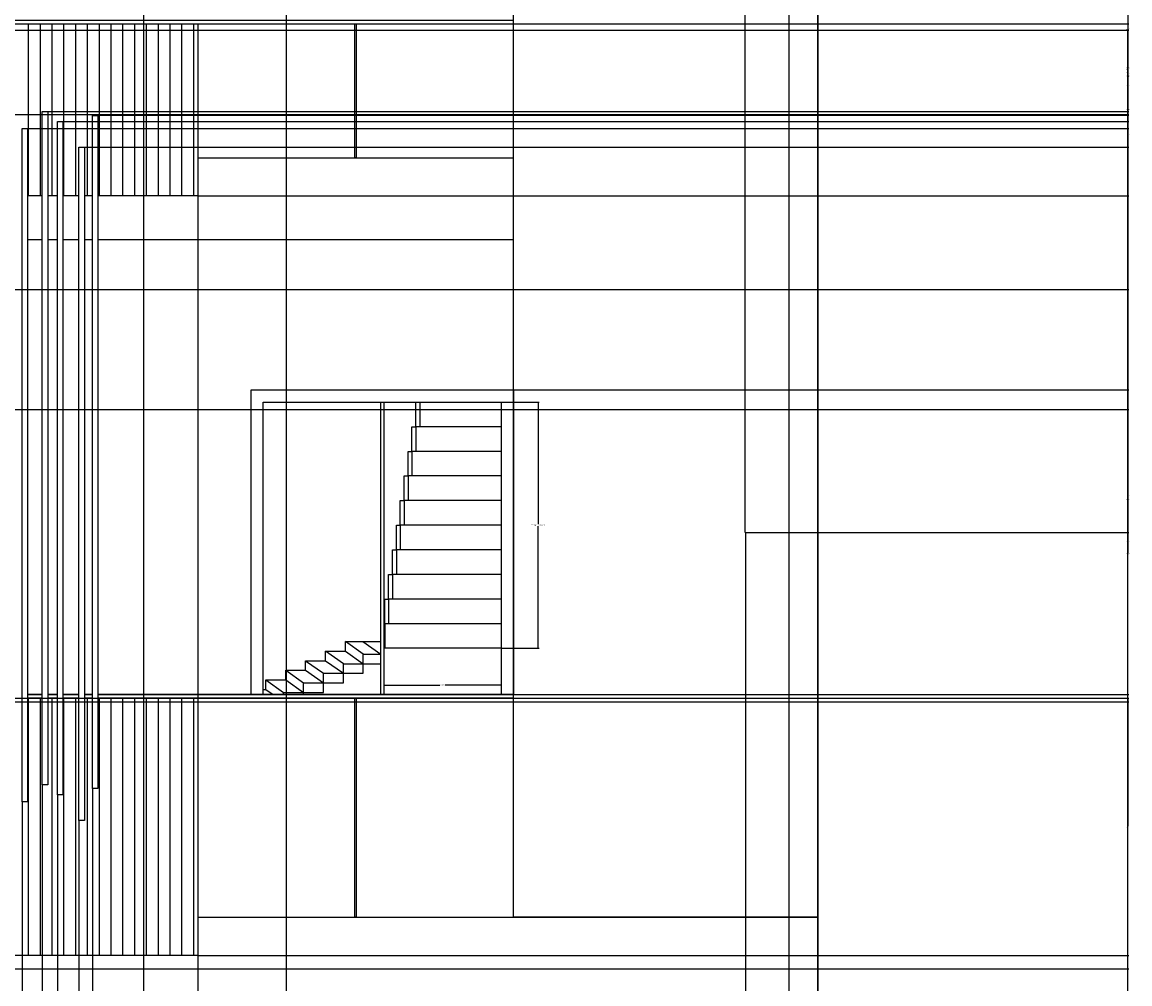
# Model space of a CAD drawing. Units: feet. Extents: x 2193 to 3502, y 890 to 1601.
# Tile 14 of 17: x 3281 to 3502, y 1076 to 1268. Entities that reach past the tile are written whole.
import ezdxf

# ---------------------------------------------------------------- set-up
doc = ezdxf.new("R2010")
doc.units = ezdxf.units.FT
doc.layers.add('A-ANNO-DIMS', color=2, linetype='Continuous', lineweight=18)
doc.layers.add('A-ELEV', color=7, linetype='Continuous', lineweight=25)
doc.styles.get("Standard").update_dxf_attribs({"font": 'arial.ttf'})
doc.dimstyles.get("Standard").update_dxf_attribs({"dimtxt": 0.18, "dimasz": 0.18, "dimexe": 0.18, "dimexo": 0.0625, "dimgap": 0.09, "dimtad": 0, "dimtih": 1, "dimtoh": 1, "dimdec": 0, "dimzin": 0, "dimdsep": 46, "dimlunit": 3, "dimtxsty": 'Standard', "dimcen": 0.09, "dimadec": 0, "dimazin": 0, "dimtfac": 1, "dimtdec": 0, "dimtofl": 0, "dimtmove": 0, "dimatfit": 3, "dimfxl": 1, "dimtolj": 1, "dimtzin": 0, "dimarcsym": 0})

# ---------------------------------------------------------------- blocks, each defined once
blk = doc.blocks.new('STAIR-RAIL-B')
for p, q in [((6.38, 44.29), (6.38, 49.22)), ((5.61, 39.37), (5.61, 44.29)), ((5.61, 44.29), (6.38, 44.29)), ((23.45, 44.29), (6.38, 44.29)), ((6.38, 44.29), (6.38, 39.37)), ((4.83, 34.45), (4.83, 39.37)), ((4.83, 39.37), (5.61, 39.37)), ((23.45, 39.37), (5.61, 39.37)), ((5.61, 39.37), (5.61, 34.45)), ((4.05, 29.53), (4.05, 34.45)), ((4.05, 34.45), (4.83, 34.45)), ((23.45, 34.45), (4.83, 34.45)), ((4.83, 34.45), (4.83, 29.53)), ((3.27, 24.61), (3.27, 29.53)), ((3.27, 29.53), (4.05, 29.53)), ((23.45, 29.53), (4.05, 29.53)), ((4.05, 29.53), (4.05, 24.61)), ((2.49, 19.69), (2.49, 24.61)), ((2.49, 24.61), (3.27, 24.61)), ((23.45, 24.61), (3.27, 24.61)), ((3.27, 24.61), (3.27, 19.69)), ((1.71, 14.77), (1.71, 19.69)), ((1.71, 19.69), (2.49, 19.69)), ((23.45, 19.69), (2.49, 19.69)), ((2.49, 19.69), (2.49, 14.77)), ((0.93, 9.84), (0.93, 14.77)), ((0.93, 14.77), (1.71, 14.77)), ((23.45, 14.77), (1.71, 14.77)), ((1.71, 14.77), (1.71, 9.84)), ((0.15, 4.92), (0.15, 9.84)), ((0.15, 9.84), (0.93, 9.84)), ((23.45, 9.84), (0.93, 9.84)), ((0.93, 9.84), (0.93, 4.92)), ((23.45, 4.92), (0, 4.92)), ((0.15, 4.92), (0.15, 0)), ((23.45, 0), (0, 0))]:
    blk.add_line(p, q)
blk = doc.blocks.new('*D9')
at = {"layer": 'A-ANNO-DIMS', "color": 0, "lineweight": -2, "transparency": 16777216}
for p, q in [((3376.47, 1192.33), (3383.97, 1192.33)), ((3383.79, 1192.15), (3383.79, 1167.9)), ((3383.79, 1143.29), (3383.79, 1167.54)), ((3376.47, 1143.11), (3383.97, 1143.11))]:
    blk.add_line(p, q, dxfattribs=at)
at = {"layer": 'A-ANNO-DIMS', "color": 0, "transparency": 16777216}
for points in [[(3383.76, 1192.15), (3383.82, 1192.15), (3383.79, 1192.33)], [(3383.76, 1143.29), (3383.82, 1143.29), (3383.79, 1143.11)]]:
    blk.add_solid(points, dxfattribs=at)
at = {"layer": 'Defpoints', "color": 0, "transparency": 16777216}
for p in [(3376.4, 1192.33), (3383.79, 1192.33), (3376.4, 1143.11)]:
    blk.add_point(p, dxfattribs=at)
at = {"layer": 'A-ANNO-DIMS', "color": 0, "transparency": 16777216, "insert": (3383.79, 1167.72), "char_height": 0.18, "attachment_point": 5}
blk.add_mtext('\\A1;STAIR RAILING B 49 TYP.', dxfattribs=at)
blk = doc.blocks.new('*D10')
at = {"layer": 'A-ANNO-DIMS', "color": 0, "lineweight": -2, "transparency": 16777216}
for p, q in [((3352.95, 1143.05), (3352.95, 1135.55)), ((3376.4, 1143.05), (3376.4, 1135.55)), ((3353.13, 1135.73), (3364.15, 1135.73)), ((3376.22, 1135.73), (3365.21, 1135.73))]:
    blk.add_line(p, q, dxfattribs=at)
at = {"layer": 'A-ANNO-DIMS', "color": 0, "transparency": 16777216}
for points in [[(3353.13, 1135.76), (3353.13, 1135.7), (3352.95, 1135.73)], [(3376.22, 1135.76), (3376.22, 1135.7), (3376.4, 1135.73)]]:
    blk.add_solid(points, dxfattribs=at)
at = {"layer": 'Defpoints', "color": 0, "transparency": 16777216}
for p in [(3352.95, 1143.11), (3376.4, 1143.11), (3376.4, 1135.73)]:
    blk.add_point(p, dxfattribs=at)
at = {"layer": 'A-ANNO-DIMS', "color": 0, "transparency": 16777216, "insert": (3364.68, 1135.73), "char_height": 0.18, "attachment_point": 5}
blk.add_mtext('\\A1;23 TYP.', dxfattribs=at)
blk = doc.blocks.new('*D13')
at = {"layer": 'A-ANNO-DIMS', "color": 0, "lineweight": -2, "transparency": 16777216}
for p, q in [((2934.37, 950.89), (2934.37, 1601.47)), ((2934.55, 1601.29), (3186.64, 1601.29)), ((3439.51, 1601.29), (3187.43, 1601.29)), ((3439.69, 1541.11), (3439.69, 1601.47))]:
    blk.add_line(p, q, dxfattribs=at)
at = {"layer": 'A-ANNO-DIMS', "color": 0, "transparency": 16777216}
for points in [[(2934.55, 1601.32), (2934.55, 1601.26), (2934.37, 1601.29)], [(3439.51, 1601.32), (3439.51, 1601.26), (3439.69, 1601.29)]]:
    blk.add_solid(points, dxfattribs=at)
at = {"layer": 'Defpoints', "color": 0, "transparency": 16777216}
for p in [(3439.69, 1601.29), (3439.69, 1541.04), (2934.37, 950.82)]:
    blk.add_point(p, dxfattribs=at)
at = {"layer": 'A-ANNO-DIMS', "color": 0, "transparency": 16777216, "insert": (3187.03, 1601.29), "char_height": 0.18, "attachment_point": 5}
blk.add_mtext('\\A1;505.3', dxfattribs=at)
blk = doc.blocks.new('*D18')
at = {"layer": 'A-ANNO-DIMS', "color": 0, "lineweight": -2, "transparency": 16777216}
for p, q in [((3439.75, 1541.04), (3501.85, 1541.04)), ((3501.67, 1540.86), (3501.67, 1246.12)), ((3501.67, 951), (3501.67, 1245.75)), ((3441.48, 950.82), (3501.85, 950.82))]:
    blk.add_line(p, q, dxfattribs=at)
at = {"layer": 'A-ANNO-DIMS', "color": 0, "transparency": 16777216}
for points in [[(3501.64, 1540.86), (3501.7, 1540.86), (3501.67, 1541.04)], [(3501.64, 951), (3501.7, 951), (3501.67, 950.82)]]:
    blk.add_solid(points, dxfattribs=at)
at = {"layer": 'Defpoints', "color": 0, "transparency": 16777216}
for p in [(3439.69, 1541.04), (3501.67, 1541.04), (3441.42, 950.82)]:
    blk.add_point(p, dxfattribs=at)
at = {"layer": 'A-ANNO-DIMS', "color": 0, "transparency": 16777216, "insert": (3501.67, 1245.93), "char_height": 0.18, "attachment_point": 5}
blk.add_mtext('\\A1;590.2', dxfattribs=at)
blk = doc.blocks.new('*D31')
at = {"layer": 'A-ANNO-DIMS', "color": 0, "lineweight": -2, "transparency": 16777216}
for p, q in [((2760.54, 1541.04), (3501.85, 1541.04)), ((3501.67, 1540.86), (3501.67, 1246.12)), ((3501.67, 951), (3501.67, 1245.75)), ((2762.27, 950.82), (3501.85, 950.82))]:
    blk.add_line(p, q, dxfattribs=at)
at = {"layer": 'A-ANNO-DIMS', "color": 0, "transparency": 16777216}
for points in [[(3501.64, 1540.86), (3501.7, 1540.86), (3501.67, 1541.04)], [(3501.64, 951), (3501.7, 951), (3501.67, 950.82)]]:
    blk.add_solid(points, dxfattribs=at)
at = {"layer": 'Defpoints', "color": 0, "transparency": 16777216}
for p in [(2760.47, 1541.04), (3501.67, 1541.04), (2762.2, 950.82)]:
    blk.add_point(p, dxfattribs=at)
at = {"layer": 'A-ANNO-DIMS', "color": 0, "transparency": 16777216, "insert": (3501.67, 1245.93), "char_height": 0.18, "attachment_point": 5}
blk.add_mtext('\\A1;590.2', dxfattribs=at)
blk = doc.blocks.new('*D62')
at = {"layer": 'A-ANNO-DIMS', "color": 0, "lineweight": -2, "transparency": 16777216}
for p, q in [((2974.18, 1266.71), (3501.85, 1266.71)), ((3501.67, 1266.53), (3501.67, 1173.05)), ((3501.67, 1079.21), (3501.67, 1172.69)), ((2974.18, 1079.03), (3501.85, 1079.03))]:
    blk.add_line(p, q, dxfattribs=at)
at = {"layer": 'A-ANNO-DIMS', "color": 0, "transparency": 16777216}
for points in [[(3501.64, 1266.53), (3501.7, 1266.53), (3501.67, 1266.71)], [(3501.64, 1079.21), (3501.7, 1079.21), (3501.67, 1079.03)]]:
    blk.add_solid(points, dxfattribs=at)
at = {"layer": 'Defpoints', "color": 0, "transparency": 16777216}
for p in [(2974.12, 1266.71), (3501.67, 1266.71), (2974.12, 1079.03)]:
    blk.add_point(p, dxfattribs=at)
at = {"layer": 'A-ANNO-DIMS', "color": 0, "transparency": 16777216, "insert": (3501.67, 1172.87), "char_height": 0.18, "attachment_point": 5}
blk.add_mtext('\\A1;187.68', dxfattribs=at)
blk = doc.blocks.new('*D67')
at = {"layer": 'A-ANNO-DIMS', "color": 0, "lineweight": -2, "transparency": 16777216}
for p, q in [((2980.78, 1214.84), (3501.85, 1214.84)), ((3501.67, 1214.66), (3501.67, 1173.8)), ((3501.67, 1132.57), (3501.67, 1173.43)), ((2980.78, 1132.39), (3501.85, 1132.39))]:
    blk.add_line(p, q, dxfattribs=at)
at = {"layer": 'A-ANNO-DIMS', "color": 0, "transparency": 16777216}
for points in [[(3501.64, 1214.66), (3501.7, 1214.66), (3501.67, 1214.84)], [(3501.64, 1132.57), (3501.7, 1132.57), (3501.67, 1132.39)]]:
    blk.add_solid(points, dxfattribs=at)
at = {"layer": 'Defpoints', "color": 0, "transparency": 16777216}
for p in [(2980.72, 1214.84), (3501.67, 1214.84), (2980.72, 1132.39)]:
    blk.add_point(p, dxfattribs=at)
at = {"layer": 'A-ANNO-DIMS', "color": 0, "transparency": 16777216, "insert": (3501.67, 1173.62), "char_height": 0.18, "attachment_point": 5}
blk.add_mtext('\\A1;82.44', dxfattribs=at)
blk = doc.blocks.new('*D69')
at = {"layer": 'A-ANNO-DIMS', "color": 0, "lineweight": -2, "transparency": 16777216}
for p, q in [((3425.25, 1367.57), (3501.85, 1367.57)), ((3501.67, 1367.39), (3501.67, 1267.09)), ((3501.67, 1166.41), (3501.67, 1266.72)), ((3425.25, 1166.23), (3501.85, 1166.23))]:
    blk.add_line(p, q, dxfattribs=at)
at = {"layer": 'A-ANNO-DIMS', "color": 0, "transparency": 16777216}
for points in [[(3501.64, 1367.39), (3501.7, 1367.39), (3501.67, 1367.57)], [(3501.64, 1166.41), (3501.7, 1166.41), (3501.67, 1166.23)]]:
    blk.add_solid(points, dxfattribs=at)
at = {"layer": 'Defpoints', "color": 0, "transparency": 16777216}
for p in [(3425.19, 1367.57), (3501.67, 1367.57), (3425.19, 1166.23)]:
    blk.add_point(p, dxfattribs=at)
at = {"layer": 'A-ANNO-DIMS', "color": 0, "transparency": 16777216, "insert": (3501.67, 1266.9), "char_height": 0.18, "attachment_point": 5}
blk.add_mtext('\\A1;201.34', dxfattribs=at)
blk = doc.blocks.new('*D70')
at = {"layer": 'A-ANNO-DIMS', "color": 0, "lineweight": -2, "transparency": 16777216}
for p, q in [((3425.19, 1166.17), (3425.19, 890.39)), ((3439.69, 1166.17), (3439.69, 890.39)), ((3425.37, 890.57), (3431.98, 890.57)), ((3439.51, 890.57), (3432.89, 890.57))]:
    blk.add_line(p, q, dxfattribs=at)
at = {"layer": 'A-ANNO-DIMS', "color": 0, "transparency": 16777216}
for points in [[(3425.37, 890.6), (3425.37, 890.54), (3425.19, 890.57)], [(3439.51, 890.6), (3439.51, 890.54), (3439.69, 890.57)]]:
    blk.add_solid(points, dxfattribs=at)
at = {"layer": 'Defpoints', "color": 0, "transparency": 16777216}
for p in [(3425.19, 1166.23), (3439.69, 1166.23), (3439.69, 890.57)]:
    blk.add_point(p, dxfattribs=at)
at = {"layer": 'A-ANNO-DIMS', "color": 0, "transparency": 16777216, "insert": (3432.44, 890.57), "char_height": 0.18, "attachment_point": 5}
blk.add_mtext('\\A1;14.502', dxfattribs=at)
blk = doc.blocks.new('*D76')
at = {"layer": 'A-ANNO-DIMS', "color": 0, "lineweight": -2, "transparency": 16777216}
for p, q in [((3259.05, 1190.87), (3501.85, 1190.87)), ((3501.67, 1190.69), (3501.67, 1162.17)), ((3501.67, 1133.29), (3501.67, 1161.81)), ((3259.52, 1133.11), (3501.85, 1133.11))]:
    blk.add_line(p, q, dxfattribs=at)
at = {"layer": 'A-ANNO-DIMS', "color": 0, "transparency": 16777216}
for points in [[(3501.64, 1190.69), (3501.7, 1190.69), (3501.67, 1190.87)], [(3501.64, 1133.29), (3501.7, 1133.29), (3501.67, 1133.11)]]:
    blk.add_solid(points, dxfattribs=at)
at = {"layer": 'Defpoints', "color": 0, "transparency": 16777216}
for p in [(3258.98, 1190.87), (3501.67, 1190.87), (3259.46, 1133.11)]:
    blk.add_point(p, dxfattribs=at)
at = {"layer": 'A-ANNO-DIMS', "color": 0, "transparency": 16777216, "insert": (3501.67, 1161.99), "char_height": 0.18, "attachment_point": 5}
blk.add_mtext('\\A1;57.75', dxfattribs=at)
blk = doc.blocks.new('*D79')
at = {"layer": 'A-ANNO-DIMS', "color": 0, "lineweight": -2, "transparency": 16777216}
for p, q in [((3326.46, 1194.77), (3501.85, 1194.77)), ((3501.67, 1194.59), (3501.67, 1164.5)), ((3501.67, 1134.04), (3501.67, 1164.13)), ((3326.46, 1133.86), (3501.85, 1133.86))]:
    blk.add_line(p, q, dxfattribs=at)
at = {"layer": 'A-ANNO-DIMS', "color": 0, "transparency": 16777216}
for points in [[(3501.64, 1194.59), (3501.7, 1194.59), (3501.67, 1194.77)], [(3501.64, 1134.04), (3501.7, 1134.04), (3501.67, 1133.86)]]:
    blk.add_solid(points, dxfattribs=at)
at = {"layer": 'Defpoints', "color": 0, "transparency": 16777216}
for p in [(3326.4, 1194.77), (3501.67, 1194.77), (3326.4, 1133.86)]:
    blk.add_point(p, dxfattribs=at)
at = {"layer": 'A-ANNO-DIMS', "color": 0, "transparency": 16777216, "insert": (3501.67, 1164.31), "char_height": 0.18, "attachment_point": 5}
blk.add_mtext('\\A1;60.92', dxfattribs=at)
blk = doc.blocks.new('*D80')
at = {"layer": 'A-ANNO-DIMS', "color": 0, "lineweight": -2, "transparency": 16777216}
for p, q in [((3198.15, 1233.5), (3198.15, 890.39)), ((3315.74, 1233.5), (3315.74, 890.39)), ((3198.33, 890.57), (3256.49, 890.57)), ((3315.56, 890.57), (3257.4, 890.57))]:
    blk.add_line(p, q, dxfattribs=at)
at = {"layer": 'A-ANNO-DIMS', "color": 0, "transparency": 16777216}
for points in [[(3198.33, 890.6), (3198.33, 890.54), (3198.15, 890.57)], [(3315.56, 890.6), (3315.56, 890.54), (3315.74, 890.57)]]:
    blk.add_solid(points, dxfattribs=at)
at = {"layer": 'Defpoints', "color": 0, "transparency": 16777216}
for p in [(3198.15, 1233.56), (3315.74, 1233.56), (3315.74, 890.57)]:
    blk.add_point(p, dxfattribs=at)
at = {"layer": 'A-ANNO-DIMS', "color": 0, "transparency": 16777216, "insert": (3256.94, 890.57), "char_height": 0.18, "attachment_point": 5}
blk.add_mtext('\\A1;117.58', dxfattribs=at)
blk = doc.blocks.new('*D81')
at = {"layer": 'A-ANNO-DIMS', "color": 0, "lineweight": -2, "transparency": 16777216}
for p, q in [((3315.8, 1267.92), (3501.85, 1267.92)), ((3501.67, 1267.74), (3501.67, 1250.92)), ((3501.67, 1233.74), (3501.67, 1250.56)), ((3315.8, 1233.56), (3501.85, 1233.56))]:
    blk.add_line(p, q, dxfattribs=at)
at = {"layer": 'A-ANNO-DIMS', "color": 0, "transparency": 16777216}
for points in [[(3501.64, 1267.74), (3501.7, 1267.74), (3501.67, 1267.92)], [(3501.64, 1233.74), (3501.7, 1233.74), (3501.67, 1233.56)]]:
    blk.add_solid(points, dxfattribs=at)
at = {"layer": 'Defpoints', "color": 0, "transparency": 16777216}
for p in [(3315.74, 1267.92), (3501.67, 1267.92), (3315.74, 1233.56)]:
    blk.add_point(p, dxfattribs=at)
at = {"layer": 'A-ANNO-DIMS', "color": 0, "transparency": 16777216, "insert": (3501.67, 1250.74), "char_height": 0.18, "attachment_point": 5}
blk.add_mtext('\\A1;34.356', dxfattribs=at)
blk = doc.blocks.new('*D82')
at = {"layer": 'A-ANNO-DIMS', "color": 0, "lineweight": -2, "transparency": 16777216}
for p, q in [((3315.8, 1133.11), (3501.85, 1133.11)), ((3501.67, 1132.93), (3501.67, 1107.6)), ((3501.67, 1081.91), (3501.67, 1107.24)), ((3315.8, 1081.73), (3501.85, 1081.73))]:
    blk.add_line(p, q, dxfattribs=at)
at = {"layer": 'A-ANNO-DIMS', "color": 0, "transparency": 16777216}
for points in [[(3501.64, 1132.93), (3501.7, 1132.93), (3501.67, 1133.11)], [(3501.64, 1081.91), (3501.7, 1081.91), (3501.67, 1081.73)]]:
    blk.add_solid(points, dxfattribs=at)
at = {"layer": 'Defpoints', "color": 0, "transparency": 16777216}
for p in [(3315.74, 1133.11), (3501.67, 1133.11), (3315.74, 1081.73)]:
    blk.add_point(p, dxfattribs=at)
at = {"layer": 'A-ANNO-DIMS', "color": 0, "transparency": 16777216, "insert": (3501.67, 1107.42), "char_height": 0.18, "attachment_point": 5}
blk.add_mtext('\\A1;51.39', dxfattribs=at)
blk = doc.blocks.new('*D86')
at = {"layer": 'A-ANNO-DIMS', "color": 0, "lineweight": -2, "transparency": 16777216}
for p, q in [((3277.81, 1115.17), (3277.81, 890.39)), ((3280.64, 1112.39), (3280.64, 890.39)), ((3277.99, 890.57), (3278.83, 890.57)), ((3280.46, 890.57), (3279.62, 890.57))]:
    blk.add_line(p, q, dxfattribs=at)
at = {"layer": 'A-ANNO-DIMS', "color": 0, "transparency": 16777216}
for points in [[(3277.99, 890.6), (3277.99, 890.54), (3277.81, 890.57)], [(3280.46, 890.6), (3280.46, 890.54), (3280.64, 890.57)]]:
    blk.add_solid(points, dxfattribs=at)
at = {"layer": 'Defpoints', "color": 0, "transparency": 16777216}
for p in [(3277.81, 1115.23), (3280.64, 1112.45), (3280.64, 890.57)]:
    blk.add_point(p, dxfattribs=at)
at = {"layer": 'A-ANNO-DIMS', "color": 0, "transparency": 16777216, "insert": (3279.22, 890.57), "char_height": 0.18, "attachment_point": 5}
blk.add_mtext('\\A1;2.832', dxfattribs=at)
blk = doc.blocks.new('*D87')
at = {"layer": 'A-ANNO-DIMS', "color": 0, "lineweight": -2, "transparency": 16777216}
for p, q in [((3284.65, 1115.79), (3284.65, 890.39)), ((3280.64, 1112.39), (3280.64, 890.39)), ((3280.82, 890.57), (3282.27, 890.57)), ((3284.47, 890.57), (3283.03, 890.57))]:
    blk.add_line(p, q, dxfattribs=at)
at = {"layer": 'A-ANNO-DIMS', "color": 0, "transparency": 16777216}
for points in [[(3280.82, 890.6), (3280.82, 890.54), (3280.64, 890.57)], [(3284.47, 890.6), (3284.47, 890.54), (3284.65, 890.57)]]:
    blk.add_solid(points, dxfattribs=at)
at = {"layer": 'Defpoints', "color": 0, "transparency": 16777216}
for p in [(3284.65, 1115.85), (3280.64, 1112.45), (3284.65, 890.57)]:
    blk.add_point(p, dxfattribs=at)
at = {"layer": 'A-ANNO-DIMS', "color": 0, "transparency": 16777216, "insert": (3282.65, 890.57), "char_height": 0.18, "attachment_point": 5}
blk.add_mtext('\\A1;4.011', dxfattribs=at)
blk = doc.blocks.new('*D88')
at = {"layer": 'A-ANNO-DIMS', "color": 0, "lineweight": -2, "transparency": 16777216}
for p, q in [((3284.65, 1115.79), (3284.65, 890.39)), ((3287.7, 1113.78), (3287.7, 890.39)), ((3284.83, 890.57), (3285.78, 890.57)), ((3287.52, 890.57), (3286.57, 890.57))]:
    blk.add_line(p, q, dxfattribs=at)
at = {"layer": 'A-ANNO-DIMS', "color": 0, "transparency": 16777216}
for points in [[(3284.83, 890.6), (3284.83, 890.54), (3284.65, 890.57)], [(3287.52, 890.6), (3287.52, 890.54), (3287.7, 890.57)]]:
    blk.add_solid(points, dxfattribs=at)
at = {"layer": 'Defpoints', "color": 0, "transparency": 16777216}
for p in [(3284.65, 1115.85), (3287.7, 1113.84), (3287.7, 890.57)]:
    blk.add_point(p, dxfattribs=at)
at = {"layer": 'A-ANNO-DIMS', "color": 0, "transparency": 16777216, "insert": (3286.18, 890.57), "char_height": 0.18, "attachment_point": 5}
blk.add_mtext('\\A1;3.052', dxfattribs=at)
blk = doc.blocks.new('*D89')
at = {"layer": 'A-ANNO-DIMS', "color": 0, "lineweight": -2, "transparency": 16777216}
for p, q in [((3287.7, 1113.78), (3287.7, 890.39)), ((3291.98, 1108.64), (3291.98, 890.39)), ((3287.88, 890.57), (3289.44, 890.57)), ((3291.8, 890.57), (3290.24, 890.57))]:
    blk.add_line(p, q, dxfattribs=at)
at = {"layer": 'A-ANNO-DIMS', "color": 0, "transparency": 16777216}
for points in [[(3287.88, 890.6), (3287.88, 890.54), (3287.7, 890.57)], [(3291.8, 890.6), (3291.8, 890.54), (3291.98, 890.57)]]:
    blk.add_solid(points, dxfattribs=at)
at = {"layer": 'Defpoints', "color": 0, "transparency": 16777216}
for p in [(3287.7, 1113.84), (3291.98, 1108.7), (3291.98, 890.57)]:
    blk.add_point(p, dxfattribs=at)
at = {"layer": 'A-ANNO-DIMS', "color": 0, "transparency": 16777216, "insert": (3289.84, 890.57), "char_height": 0.18, "attachment_point": 5}
blk.add_mtext('\\A1;4.273', dxfattribs=at)
blk = doc.blocks.new('*D90')
at = {"layer": 'A-ANNO-DIMS', "color": 0, "lineweight": -2, "transparency": 16777216}
for p, q in [((3294.68, 1115), (3294.68, 890.39)), ((3291.98, 1108.64), (3291.98, 890.39)), ((3292.16, 890.57), (3292.93, 890.57)), ((3294.5, 890.57), (3293.72, 890.57))]:
    blk.add_line(p, q, dxfattribs=at)
at = {"layer": 'A-ANNO-DIMS', "color": 0, "transparency": 16777216}
for points in [[(3292.16, 890.6), (3292.16, 890.54), (3291.98, 890.57)], [(3294.5, 890.6), (3294.5, 890.54), (3294.68, 890.57)]]:
    blk.add_solid(points, dxfattribs=at)
at = {"layer": 'Defpoints', "color": 0, "transparency": 16777216}
for p in [(3294.68, 1115.06), (3291.98, 1108.7), (3294.68, 890.57)]:
    blk.add_point(p, dxfattribs=at)
at = {"layer": 'A-ANNO-DIMS', "color": 0, "transparency": 16777216, "insert": (3293.33, 890.57), "char_height": 0.18, "attachment_point": 5}
blk.add_mtext('\\A1;2.703', dxfattribs=at)
blk = doc.blocks.new('*D91')
at = {"layer": 'A-ANNO-DIMS', "color": 0, "lineweight": -2, "transparency": 16777216}
for p, q in [((3277.2, 1267.92), (3501.85, 1267.92)), ((3501.67, 1267.74), (3501.67, 1259.05)), ((3501.67, 1250.01), (3501.67, 1258.69)), ((3277.87, 1249.83), (3501.85, 1249.83))]:
    blk.add_line(p, q, dxfattribs=at)
at = {"layer": 'A-ANNO-DIMS', "color": 0, "transparency": 16777216}
for points in [[(3501.64, 1267.74), (3501.7, 1267.74), (3501.67, 1267.92)], [(3501.64, 1250.01), (3501.7, 1250.01), (3501.67, 1249.83)]]:
    blk.add_solid(points, dxfattribs=at)
at = {"layer": 'Defpoints', "color": 0, "transparency": 16777216}
for p in [(3277.14, 1267.92), (3501.67, 1267.92), (3277.81, 1249.83)]:
    blk.add_point(p, dxfattribs=at)
at = {"layer": 'A-ANNO-DIMS', "color": 0, "transparency": 16777216, "insert": (3501.67, 1258.87), "char_height": 0.18, "attachment_point": 5}
blk.add_mtext('\\A1;18.09', dxfattribs=at)
blk = doc.blocks.new('*D92')
at = {"layer": 'A-ANNO-DIMS', "color": 0, "lineweight": -2, "transparency": 16777216}
for p, q in [((3281.92, 1267.92), (3501.85, 1267.92)), ((3501.67, 1267.74), (3501.67, 1257.66)), ((3501.67, 1247.22), (3501.67, 1257.3)), ((3280.7, 1247.04), (3501.85, 1247.04))]:
    blk.add_line(p, q, dxfattribs=at)
at = {"layer": 'A-ANNO-DIMS', "color": 0, "transparency": 16777216}
for points in [[(3501.64, 1267.74), (3501.7, 1267.74), (3501.67, 1267.92)], [(3501.64, 1247.22), (3501.7, 1247.22), (3501.67, 1247.04)]]:
    blk.add_solid(points, dxfattribs=at)
at = {"layer": 'Defpoints', "color": 0, "transparency": 16777216}
for p in [(3281.86, 1267.92), (3501.67, 1267.92), (3280.64, 1247.04)]:
    blk.add_point(p, dxfattribs=at)
at = {"layer": 'A-ANNO-DIMS', "color": 0, "transparency": 16777216, "insert": (3501.67, 1257.48), "char_height": 0.18, "attachment_point": 5}
blk.add_mtext('\\A1;20.875', dxfattribs=at)
blk = doc.blocks.new('*D93')
at = {"layer": 'A-ANNO-DIMS', "color": 0, "lineweight": -2, "transparency": 16777216}
for p, q in [((3284.28, 1267.92), (3501.85, 1267.92)), ((3501.67, 1267.74), (3501.67, 1259.36)), ((3501.67, 1250.62), (3501.67, 1259)), ((3284.71, 1250.44), (3501.85, 1250.44))]:
    blk.add_line(p, q, dxfattribs=at)
at = {"layer": 'A-ANNO-DIMS', "color": 0, "transparency": 16777216}
for points in [[(3501.64, 1267.74), (3501.7, 1267.74), (3501.67, 1267.92)], [(3501.64, 1250.62), (3501.7, 1250.62), (3501.67, 1250.44)]]:
    blk.add_solid(points, dxfattribs=at)
at = {"layer": 'Defpoints', "color": 0, "transparency": 16777216}
for p in [(3284.22, 1267.92), (3501.67, 1267.92), (3284.65, 1250.44)]:
    blk.add_point(p, dxfattribs=at)
at = {"layer": 'A-ANNO-DIMS', "color": 0, "transparency": 16777216, "insert": (3501.67, 1259.18), "char_height": 0.18, "attachment_point": 5}
blk.add_mtext('\\A1;17.477', dxfattribs=at)
blk = doc.blocks.new('*D94')
at = {"layer": 'A-ANNO-DIMS', "color": 0, "lineweight": -2, "transparency": 16777216}
for p, q in [((3288.99, 1267.92), (3501.85, 1267.92)), ((3501.67, 1267.74), (3501.67, 1258.36)), ((3501.67, 1248.62), (3501.67, 1257.99)), ((3287.77, 1248.44), (3501.85, 1248.44))]:
    blk.add_line(p, q, dxfattribs=at)
at = {"layer": 'A-ANNO-DIMS', "color": 0, "transparency": 16777216}
for points in [[(3501.64, 1267.74), (3501.7, 1267.74), (3501.67, 1267.92)], [(3501.64, 1248.62), (3501.7, 1248.62), (3501.67, 1248.44)]]:
    blk.add_solid(points, dxfattribs=at)
at = {"layer": 'Defpoints', "color": 0, "transparency": 16777216}
for p in [(3288.93, 1267.92), (3501.67, 1267.92), (3287.7, 1248.44)]:
    blk.add_point(p, dxfattribs=at)
at = {"layer": 'A-ANNO-DIMS', "color": 0, "transparency": 16777216, "insert": (3501.67, 1258.18), "char_height": 0.18, "attachment_point": 5}
blk.add_mtext('\\A1;19.48', dxfattribs=at)
blk = doc.blocks.new('*D95')
at = {"layer": 'A-ANNO-DIMS', "color": 0, "lineweight": -2, "transparency": 16777216}
for p, q in [((3291.35, 1267.92), (3501.85, 1267.92)), ((3501.67, 1267.74), (3501.67, 1255.79)), ((3501.67, 1243.48), (3501.67, 1255.42)), ((3292.04, 1243.3), (3501.85, 1243.3))]:
    blk.add_line(p, q, dxfattribs=at)
at = {"layer": 'A-ANNO-DIMS', "color": 0, "transparency": 16777216}
for points in [[(3501.64, 1267.74), (3501.7, 1267.74), (3501.67, 1267.92)], [(3501.64, 1243.48), (3501.7, 1243.48), (3501.67, 1243.3)]]:
    blk.add_solid(points, dxfattribs=at)
at = {"layer": 'Defpoints', "color": 0, "transparency": 16777216}
for p in [(3291.29, 1267.92), (3501.67, 1267.92), (3291.98, 1243.3)]:
    blk.add_point(p, dxfattribs=at)
at = {"layer": 'A-ANNO-DIMS', "color": 0, "transparency": 16777216, "insert": (3501.67, 1255.61), "char_height": 0.18, "attachment_point": 5}
blk.add_mtext('\\A1;24.62', dxfattribs=at)
blk = doc.blocks.new('*D96')
at = {"layer": 'A-ANNO-DIMS', "color": 0, "lineweight": -2, "transparency": 16777216}
for p, q in [((3296.07, 1267.92), (3501.85, 1267.92)), ((3501.67, 1267.74), (3501.67, 1258.97)), ((3501.67, 1249.84), (3501.67, 1258.6)), ((3294.74, 1249.66), (3501.85, 1249.66))]:
    blk.add_line(p, q, dxfattribs=at)
at = {"layer": 'A-ANNO-DIMS', "color": 0, "transparency": 16777216}
for points in [[(3501.64, 1267.74), (3501.7, 1267.74), (3501.67, 1267.92)], [(3501.64, 1249.84), (3501.7, 1249.84), (3501.67, 1249.66)]]:
    blk.add_solid(points, dxfattribs=at)
at = {"layer": 'Defpoints', "color": 0, "transparency": 16777216}
for p in [(3296, 1267.92), (3501.67, 1267.92), (3294.68, 1249.66)]:
    blk.add_point(p, dxfattribs=at)
at = {"layer": 'A-ANNO-DIMS', "color": 0, "transparency": 16777216, "insert": (3501.67, 1258.79), "char_height": 0.18, "attachment_point": 5}
blk.add_mtext('\\A1;18.26', dxfattribs=at)
blk = doc.blocks.new('*D97')
at = {"layer": 'A-ANNO-DIMS', "color": 0, "lineweight": -2, "transparency": 16777216}
for p, q in [((3111.13, 1032.26), (3111.13, 1601.47)), ((3111.31, 1601.29), (3207.6, 1601.29)), ((3304.79, 1601.29), (3208.51, 1601.29)), ((3304.97, 1032.26), (3304.97, 1601.47))]:
    blk.add_line(p, q, dxfattribs=at)
at = {"layer": 'A-ANNO-DIMS', "color": 0, "transparency": 16777216}
for points in [[(3111.31, 1601.32), (3111.31, 1601.26), (3111.13, 1601.29)], [(3304.79, 1601.32), (3304.79, 1601.26), (3304.97, 1601.29)]]:
    blk.add_solid(points, dxfattribs=at)
at = {"layer": 'Defpoints', "color": 0, "transparency": 16777216}
for p in [(3304.97, 1601.29), (3111.13, 1032.19), (3304.97, 1032.19)]:
    blk.add_point(p, dxfattribs=at)
at = {"layer": 'A-ANNO-DIMS', "color": 0, "transparency": 16777216, "insert": (3208.05, 1601.29), "char_height": 0.18, "attachment_point": 5}
blk.add_mtext('\\A1;193.84', dxfattribs=at)
blk = doc.blocks.new('*D123')
at = {"layer": 'A-ANNO-DIMS', "color": 0, "lineweight": -2, "transparency": 16777216}
for p, q in [((3433.98, 1073.09), (3433.98, 1601.47)), ((3434.16, 1601.29), (3436.44, 1601.29)), ((3439.51, 1601.29), (3437.23, 1601.29)), ((3439.69, 1073.09), (3439.69, 1601.47))]:
    blk.add_line(p, q, dxfattribs=at)
at = {"layer": 'A-ANNO-DIMS', "color": 0, "transparency": 16777216}
for points in [[(3434.16, 1601.32), (3434.16, 1601.26), (3433.98, 1601.29)], [(3439.51, 1601.32), (3439.51, 1601.26), (3439.69, 1601.29)]]:
    blk.add_solid(points, dxfattribs=at)
at = {"layer": 'Defpoints', "color": 0, "transparency": 16777216}
for p in [(3439.69, 1601.29), (3433.98, 1073.03), (3439.69, 1073.03)]:
    blk.add_point(p, dxfattribs=at)
at = {"layer": 'A-ANNO-DIMS', "color": 0, "transparency": 16777216, "insert": (3436.84, 1601.29), "char_height": 0.18, "attachment_point": 5}
blk.add_mtext('\\A1;5.707', dxfattribs=at)
blk = doc.blocks.new('*D125')
at = {"layer": 'A-ANNO-DIMS', "color": 0, "lineweight": -2, "transparency": 16777216}
for p, q in [((3304.97, 1073.09), (3304.97, 1601.47)), ((3305.15, 1601.29), (3318.84, 1601.29)), ((3333.32, 1601.29), (3319.63, 1601.29)), ((3333.5, 1073.09), (3333.5, 1601.47))]:
    blk.add_line(p, q, dxfattribs=at)
at = {"layer": 'A-ANNO-DIMS', "color": 0, "transparency": 16777216}
for points in [[(3305.15, 1601.32), (3305.15, 1601.26), (3304.97, 1601.29)], [(3333.32, 1601.32), (3333.32, 1601.26), (3333.5, 1601.29)]]:
    blk.add_solid(points, dxfattribs=at)
at = {"layer": 'Defpoints', "color": 0, "transparency": 16777216}
for p in [(3333.5, 1601.29), (3304.97, 1073.03), (3333.5, 1073.03)]:
    blk.add_point(p, dxfattribs=at)
at = {"layer": 'A-ANNO-DIMS', "color": 0, "transparency": 16777216, "insert": (3319.24, 1601.29), "char_height": 0.18, "attachment_point": 5}
blk.add_mtext('\\A1;28.53', dxfattribs=at)

msp = doc.modelspace()

# ---------------------------------------------------------------- linework, layer by layer
at = {"layer": 'A-ELEV'}
for p, q in [((3439.6901, 956.8829), (3439.6901, 1494.0584)), ((3315.7352, 1241.1967), (3378.849, 1241.1967)), ((3281.7371, 1224.865), (3284.651, 1224.865)), ((3285.7483, 1224.865), (3287.703, 1224.865)), ((3288.8003, 1224.865), (3291.9757, 1224.865)), ((3293.0731, 1224.865), (3294.679, 1224.865)), ((3295.7763, 1224.865), (3378.849, 1224.865)), ((3360.1133, 1192.3273), (3360.1133, 1187.4057)), ((3425.1877, 1166.2327), (3439.6901, 1166.2327)), ((3341.2875, 1140.6364), (3341.2875, 1142.554)), ((3341.2875, 1142.554), (3345.27, 1142.554)), ((3344.8379, 1140.0352), (3341.2875, 1142.554)), ((3348.8205, 1141.9528), (3345.27, 1144.4716)), ((3345.27, 1144.4716), (3348.7495, 1144.4716)), ((3345.27, 1142.554), (3345.27, 1144.4716)), ((3345.27, 1142.554), (3348.8205, 1140.0352)), ((3348.7495, 1144.4716), (3352.2999, 1141.9528)), ((3348.7495, 1144.4716), (3352.2999, 1144.4716)), ((3337.3049, 1138.7188), (3337.3049, 1140.6364)), ((3337.3049, 1140.6364), (3341.2875, 1140.6364)), ((3337.3049, 1140.6364), (3340.8553, 1138.1177)), ((3341.2875, 1140.6364), (3344.8379, 1138.1177)), ((3348.8205, 1140.0352), (3348.8205, 1141.9528)), ((3348.8205, 1141.9528), (3352.2999, 1141.9528)), ((3333.3223, 1136.8013), (3333.3223, 1138.7188)), ((3333.3223, 1138.7188), (3337.3049, 1138.7188)), ((3333.3223, 1138.7188), (3336.8727, 1136.2001)), ((3337.3049, 1138.7188), (3340.8553, 1136.2001)), ((3340.8553, 1136.2001), (3340.8553, 1138.1177)), ((3340.8553, 1138.1177), (3344.8379, 1138.1177)), ((3344.8379, 1138.1177), (3344.8379, 1140.0352)), ((3344.8379, 1140.0352), (3348.8205, 1140.0352)), ((3344.8379, 1136.2001), (3344.8379, 1138.1177)), ((3344.8379, 1138.1177), (3348.8205, 1138.1177)), ((3348.8205, 1140.0352), (3352.2999, 1140.0352)), ((3348.8205, 1138.1177), (3348.8205, 1140.0352)), ((3329.3397, 1134.8837), (3329.3397, 1136.8013)), ((3329.3397, 1136.8013), (3333.3223, 1136.8013)), ((3329.3397, 1136.8013), (3332.8902, 1134.2825)), ((3333.3223, 1136.8013), (3336.8727, 1134.2825)), ((3336.8727, 1134.2825), (3336.8727, 1136.2001)), ((3336.8727, 1136.2001), (3340.8553, 1136.2001)), ((3340.8553, 1134.2825), (3340.8553, 1136.2001)), ((3340.8553, 1136.2001), (3344.8379, 1136.2001)), ((3328.846, 1134.8837), (3329.3397, 1134.8837)), ((3329.3397, 1134.8837), (3330.7886, 1133.8558)), ((3332.8902, 1133.8558), (3332.8902, 1134.2825)), ((3332.8902, 1134.2825), (3336.8727, 1134.2825)), ((3332.8902, 1133.8558), (3332.8902, 1133.8558)), ((3336.8727, 1133.8558), (3336.8727, 1134.2825)), ((3336.8727, 1134.2825), (3340.8553, 1134.2825)), ((3315.7352, 1089.3627), (3439.6901, 1089.3627))]:
    msp.add_line(p, q, dxfattribs=at)
for points in [[(3439.6901, 1415.3157), (3439.6901, 1089.3627), (3378.849, 1089.3627), (3378.849, 1367.5739)], [(3425.1877, 1166.2327), (3425.1877, 1367.5739)], [(3378.849, 1267.9169), (3147.5022, 1267.9169), (3147.5022, 1268.6599), (3378.849, 1268.6599)], [(3281.8579, 1267.9169), (3281.8579, 1233.561), (3281.7371, 1233.561)], [(3284.2158, 1267.9169), (3284.2158, 1233.561), (3283.0369, 1233.561)], [(3286.5736, 1267.9169), (3286.5736, 1233.561), (3285.7483, 1233.561)], [(3288.9314, 1267.9169), (3288.9314, 1233.561), (3288.8003, 1233.561)], [(3291.2893, 1267.9169), (3291.2893, 1233.561), (3290.1104, 1233.561)], [(3293.6471, 1267.9169), (3293.6471, 1233.561), (3293.0731, 1233.561)], [(3315.7352, 1267.9169), (3315.7352, 1233.561), (3295.7763, 1233.561)], [(3296.005, 1267.9169), (3296.005, 1233.561), (3295.7763, 1233.561)], [(3298.3628, 1267.9169), (3298.3628, 1233.561), (3297.1839, 1233.561)], [(3300.7206, 1267.9169), (3300.7206, 1233.561), (3299.5417, 1233.561)], [(3303.0785, 1267.9169), (3303.0785, 1233.561), (3301.8996, 1233.561)], [(3305.4363, 1267.9169), (3305.4363, 1233.561), (3304.2574, 1233.561)], [(3307.7941, 1267.9169), (3307.7941, 1233.561), (3306.6152, 1233.561)], [(3310.152, 1267.9169), (3310.152, 1233.561), (3308.9731, 1233.561)], [(3312.5098, 1267.9169), (3312.5098, 1233.561), (3311.3309, 1233.561)], [(3314.8677, 1267.9169), (3314.8677, 1233.561), (3313.6887, 1233.561)], [(3347.39, 1267.9169), (3347.39, 1241.1967), (3347.1403, 1241.1967), (3347.1403, 1267.9169)], [(3284.651, 1233.561), (3281.7371, 1233.561)], [(3287.703, 1233.561), (3285.7483, 1233.561)], [(3291.9757, 1233.561), (3288.8003, 1233.561)], [(3294.679, 1233.561), (3293.0731, 1233.561)], [(3328.846, 1133.8558), (3328.846, 1192.3273), (3376.4039, 1192.3273), (3376.4039, 1133.8558)], [(3281.7371, 1133.8558), (3284.651, 1133.8558)], [(3284.651, 1133.8558), (3281.7371, 1133.8558)], [(3285.7483, 1133.8558), (3287.703, 1133.8558)], [(3287.703, 1133.8558), (3285.7483, 1133.8558)], [(3288.8003, 1133.8558), (3291.9757, 1133.8558)], [(3291.9757, 1133.8558), (3288.8003, 1133.8558)], [(3293.0731, 1133.8558), (3294.679, 1133.8558)], [(3294.679, 1133.8558), (3293.0731, 1133.8558)], [(3378.849, 1133.8558), (3295.7763, 1133.8558)], [(3295.7763, 1133.8558), (3378.849, 1133.8558)], [(3315.7352, 1133.1128), (3315.7352, 1081.7269), (3196.9758, 1081.7269), (3196.9758, 1133.1128)], [(3281.7371, 1133.1128), (3281.8579, 1133.1128), (3281.8579, 1081.7269), (3280.679, 1081.7269)], [(3284.651, 1133.1128), (3281.7371, 1133.1128)], [(3283.0369, 1133.1128), (3284.2158, 1133.1128), (3284.2158, 1081.7269), (3283.0369, 1081.7269)], [(3285.7483, 1133.1128), (3286.5736, 1133.1128), (3286.5736, 1081.7269), (3285.3947, 1081.7269)], [(3287.703, 1133.1128), (3285.7483, 1133.1128)], [(3288.8003, 1133.1128), (3288.9314, 1133.1128), (3288.9314, 1081.7269), (3287.7525, 1081.7269)], [(3291.9757, 1133.1128), (3288.8003, 1133.1128)], [(3290.1104, 1133.1128), (3291.2893, 1133.1128), (3291.2893, 1081.7269), (3290.1104, 1081.7269)], [(3293.0731, 1133.1128), (3293.6471, 1133.1128), (3293.6471, 1081.7269), (3292.4682, 1081.7269)], [(3294.679, 1133.1128), (3293.0731, 1133.1128)], [(3295.7763, 1133.1128), (3296.005, 1133.1128), (3296.005, 1081.7269), (3294.826, 1081.7269)], [(3378.849, 1133.1128), (3295.7763, 1133.1128)], [(3297.1839, 1133.1128), (3298.3628, 1133.1128), (3298.3628, 1081.7269), (3297.1839, 1081.7269)], [(3299.5417, 1133.1128), (3300.7206, 1133.1128), (3300.7206, 1081.7269), (3299.5417, 1081.7269)], [(3301.8996, 1133.1128), (3303.0785, 1133.1128), (3303.0785, 1081.7269), (3301.8996, 1081.7269)], [(3304.2574, 1133.1128), (3305.4363, 1133.1128), (3305.4363, 1081.7269), (3304.2574, 1081.7269)], [(3306.6152, 1133.1128), (3307.7941, 1133.1128), (3307.7941, 1081.7269), (3306.6152, 1081.7269)], [(3308.9731, 1133.1128), (3310.152, 1133.1128), (3310.152, 1081.7269), (3308.9731, 1081.7269)], [(3311.3309, 1133.1128), (3312.5098, 1133.1128), (3312.5098, 1081.7269), (3311.3309, 1081.7269)], [(3313.6887, 1133.1128), (3314.8677, 1133.1128), (3314.8677, 1081.7269), (3313.6887, 1081.7269)]]:
    msp.add_lwpolyline(points, dxfattribs=at)
for points in [[(3284.651, 1250.4403), (3285.7483, 1250.4403), (3285.7483, 1115.8479), (3284.651, 1115.8479)], [(3294.679, 1249.6561), (3295.7763, 1249.6561), (3295.7763, 1115.0637), (3294.679, 1115.0637)], [(3280.6398, 1247.0422), (3281.7371, 1247.0422), (3281.7371, 1112.4498), (3280.6398, 1112.4498)], [(3287.703, 1248.4363), (3288.8003, 1248.4363), (3288.8003, 1113.8439), (3287.703, 1113.8439)], [(3291.9757, 1243.2956), (3293.0731, 1243.2956), (3293.0731, 1108.7032), (3291.9757, 1108.7032)], [(3378.849, 1133.8558), (3326.4009, 1133.8558), (3326.4009, 1194.7724), (3378.849, 1194.7724)], [(3352.2999, 1192.3273), (3352.95, 1192.3273), (3352.95, 1133.8558), (3352.2999, 1133.8558)], [(3347.1403, 1133.1128), (3347.39, 1133.1128), (3347.39, 1089.3627), (3347.1403, 1089.3627)]]:
    msp.add_lwpolyline(points, close=True, dxfattribs=at)

# ---------------------------------------------------------------- block references
msp.add_blockref('STAIR-RAIL-B', (3352.95, 1143.111), dxfattribs=at)

# ---------------------------------------------------------------- dimensions: what is measured, and where the dimension line sits
at = {"layer": 'A-ANNO-DIMS'}
for base, p1, p2, override, picture, middle in [((3439.6901, 1601.2941), (2934.3742, 950.8228), (3439.6901, 1541.0441), {"dimdec": 1, "dimlfac": 1, "dimrnd": 0, "dimzin": 0, "dimdsep": 46, "dimlunit": 2}, '*D13', (3187.0321, 1601.2941)), ((3304.9731, 1601.2941), (3111.1302, 1032.1935), (3304.9731, 1032.1935), {"dimdec": 2, "dimlfac": 1, "dimrnd": 0, "dimzin": 0, "dimdsep": 46, "dimlunit": 2}, '*D97', (3208.0516, 1601.2941)), ((3333.5009, 1601.2941), (3304.9731, 1073.031), (3333.5009, 1073.031), {"dimdec": 2, "dimlfac": 1, "dimrnd": 0, "dimzin": 0, "dimdsep": 46, "dimlunit": 2}, '*D125', (3319.237, 1601.2941)), ((3439.6901, 1601.2941), (3433.9829, 1073.031), (3439.6901, 1073.031), {"dimdec": 3, "dimlfac": 1, "dimrnd": 0, "dimzin": 0, "dimdsep": 46, "dimlunit": 2}, '*D123', (3436.8365, 1601.2941)), ((3315.7352, 890.5728), (3198.1547, 1233.561), (3315.7352, 1233.561), {"dimdec": 2, "dimlfac": 1, "dimrnd": 0, "dimzin": 0, "dimdsep": 46, "dimlunit": 2}, '*D80', (3256.9449, 890.5728)), ((3439.6901, 890.5728), (3425.1877, 1166.2327), (3439.6901, 1166.2327), {"dimdec": 3, "dimlfac": 1, "dimrnd": 0, "dimzin": 0, "dimdsep": 46, "dimlunit": 2}, '*D70', (3432.4389, 890.5728)), ((3280.6398, 890.5728), (3277.8077, 1115.2331), (3280.6398, 1112.4498), {"dimdec": 3, "dimlfac": 1, "dimrnd": 0, "dimzin": 0, "dimdsep": 46, "dimlunit": 2}, '*D86', (3279.2237, 890.5728)), ((3284.651, 890.5728), (3280.6398, 1112.4498), (3284.651, 1115.8479), {"dimdec": 3, "dimlfac": 1, "dimrnd": 0, "dimzin": 0, "dimdsep": 46, "dimlunit": 2}, '*D87', (3282.6454, 890.5728)), ((3287.703, 890.5728), (3284.651, 1115.8479), (3287.703, 1113.8439), {"dimdec": 3, "dimlfac": 1, "dimrnd": 0, "dimzin": 0, "dimdsep": 46, "dimlunit": 2}, '*D88', (3286.177, 890.5728)), ((3291.9757, 890.5728), (3287.703, 1113.8439), (3291.9757, 1108.7032), {"dimdec": 3, "dimlfac": 1, "dimrnd": 0, "dimzin": 0, "dimdsep": 46, "dimlunit": 2}, '*D89', (3289.8394, 890.5728)), ((3294.679, 890.5728), (3291.9757, 1108.7032), (3294.679, 1115.0637), {"dimdec": 3, "dimlfac": 1, "dimrnd": 0, "dimzin": 0, "dimdsep": 46, "dimlunit": 2}, '*D90', (3293.3274, 890.5728))]:
    dim = msp.add_linear_dim(base=base, p1=p1, p2=p2, dimstyle='Standard', override=override, dxfattribs=at)
    dim.commit()
    dim.dimension.update_dxf_attribs({"geometry": picture, "text_midpoint": middle})
for base, p1, p2, override, picture, middle in [((3501.6716, 1541.0441), (2762.2048, 950.8228), (2760.4733, 1541.0441), {"dimdec": 1, "dimlfac": 1, "dimrnd": 0, "dimzin": 0, "dimdsep": 46, "dimlunit": 2}, '*D31', (3501.6716, 1245.9334)), ((3501.6716, 1541.0441), (3441.4216, 950.8228), (3439.6901, 1541.0441), {"dimdec": 1, "dimlfac": 1, "dimrnd": 0, "dimzin": 0, "dimdsep": 46, "dimlunit": 2}, '*D18', (3501.6716, 1245.9334)), ((3501.6716, 1367.5739), (3425.1877, 1166.2327), (3425.1877, 1367.5739), {"dimdec": 2, "dimlfac": 1, "dimrnd": 0, "dimzin": 0, "dimdsep": 46, "dimlunit": 2}, '*D69', (3501.6716, 1266.9033)), ((3501.6716, 1266.7092), (2974.116, 1079.031), (2974.116, 1266.7092), {"dimdec": 2, "dimlfac": 1, "dimrnd": 0, "dimzin": 0, "dimdsep": 46, "dimlunit": 2}, '*D62', (3501.6716, 1172.8701)), ((3501.6716, 1267.9169), (3277.8077, 1249.8256), (3277.1423, 1267.9169), {"dimdec": 2, "dimlfac": 1, "dimrnd": 0, "dimzin": 0, "dimdsep": 46, "dimlunit": 2}, '*D91', (3501.6716, 1258.8712)), ((3501.6716, 1267.9169), (3280.6398, 1247.0422), (3281.8579, 1267.9169), {"dimdec": 3, "dimlfac": 1, "dimrnd": 0, "dimzin": 0, "dimdsep": 46, "dimlunit": 2}, '*D92', (3501.6716, 1257.4795)), ((3501.6716, 1267.9169), (3284.651, 1250.4403), (3284.2158, 1267.9169), {"dimdec": 3, "dimlfac": 1, "dimrnd": 0, "dimzin": 0, "dimdsep": 46, "dimlunit": 2}, '*D93', (3501.6716, 1259.1786)), ((3501.6716, 1267.9169), (3287.703, 1248.4363), (3288.9314, 1267.9169), {"dimdec": 2, "dimlfac": 1, "dimrnd": 0, "dimzin": 0, "dimdsep": 46, "dimlunit": 2}, '*D94', (3501.6716, 1258.1766)), ((3501.6716, 1267.9169), (3291.9757, 1243.2956), (3291.2893, 1267.9169), {"dimdec": 2, "dimlfac": 1, "dimrnd": 0, "dimzin": 0, "dimdsep": 46, "dimlunit": 2}, '*D95', (3501.6716, 1255.6062)), ((3501.6716, 1267.9169), (3294.679, 1249.6561), (3296.005, 1267.9169), {"dimdec": 2, "dimlfac": 1, "dimrnd": 0, "dimzin": 0, "dimdsep": 46, "dimlunit": 2}, '*D96', (3501.6716, 1258.7865)), ((3501.6716, 1267.9169), (3315.7352, 1233.561), (3315.7352, 1267.9169), {"dimdec": 3, "dimlfac": 1, "dimrnd": 0, "dimzin": 0, "dimdsep": 46, "dimlunit": 2}, '*D81', (3501.6716, 1250.7389)), ((3501.6716, 1214.8367), (2980.7151, 1132.3937), (2980.7151, 1214.8367), {"dimdec": 2, "dimlfac": 1, "dimrnd": 0, "dimzin": 0, "dimdsep": 46, "dimlunit": 2}, '*D67', (3501.6716, 1173.6152)), ((3501.6716, 1194.7724), (3326.4009, 1133.8558), (3326.4009, 1194.7724), {"dimdec": 2, "dimlfac": 1, "dimrnd": 0, "dimzin": 0, "dimdsep": 46, "dimlunit": 2}, '*D79', (3501.6716, 1164.3141)), ((3501.6716, 1190.8659), (3259.4585, 1133.1128), (3258.9838, 1190.8659), {"dimdec": 2, "dimlfac": 1, "dimrnd": 0, "dimzin": 0, "dimdsep": 46, "dimlunit": 2}, '*D76', (3501.6716, 1161.9893)), ((3501.6716, 1133.1128), (3315.7352, 1081.7269), (3315.7352, 1133.1128), {"dimdec": 2, "dimlfac": 1, "dimrnd": 0, "dimzin": 0, "dimdsep": 46, "dimlunit": 2}, '*D82', (3501.6716, 1107.4199))]:
    dim = msp.add_linear_dim(base=base, p1=p1, p2=p2, angle=90, dimstyle='Standard', override=override, dxfattribs=at)
    dim.commit()
    dim.dimension.update_dxf_attribs({"geometry": picture, "text_midpoint": middle})
dim = msp.add_linear_dim(base=(3383.7863, 1192.3273), p1=(3376.4039, 1143.1114), p2=(3376.4039, 1192.3273), angle=90, text='STAIR RAILING B <> TYP.', dimstyle='Standard', override={"dimdec": 0, "dimlfac": 1, "dimrnd": 0, "dimzin": 0, "dimdsep": 46, "dimlunit": 2}, dxfattribs=at)
dim.commit()
dim.dimension.update_dxf_attribs({"geometry": '*D9', "text_midpoint": (3383.7863, 1167.7194)})
dim = msp.add_linear_dim(base=(3376.4039, 1135.729), p1=(3352.95, 1143.1114), p2=(3376.4039, 1143.1114), text='<> TYP.', dimstyle='Standard', override={"dimdec": 0, "dimlfac": 1, "dimrnd": 0, "dimzin": 0, "dimdsep": 46, "dimlunit": 2}, dxfattribs=at)
dim.commit()
dim.dimension.update_dxf_attribs({"geometry": '*D10', "text_midpoint": (3364.6769, 1135.729)})

doc.saveas('drawing.dxf')
